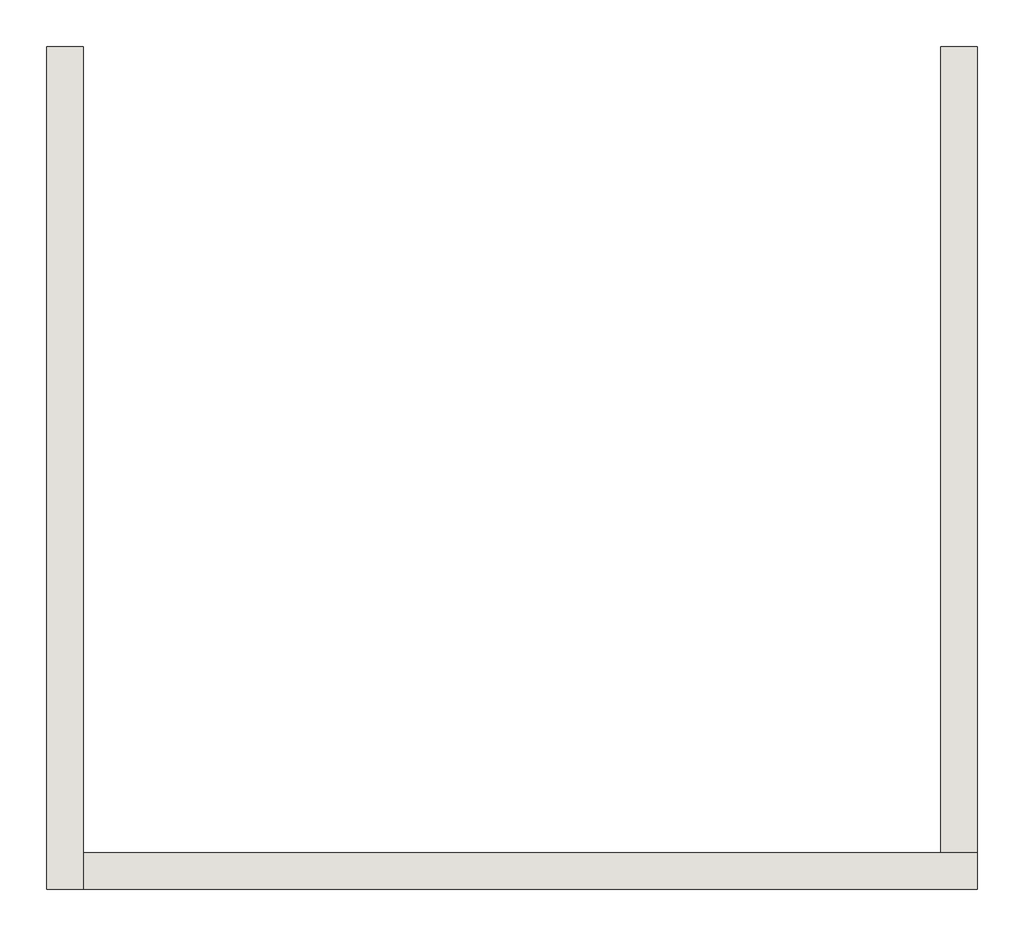
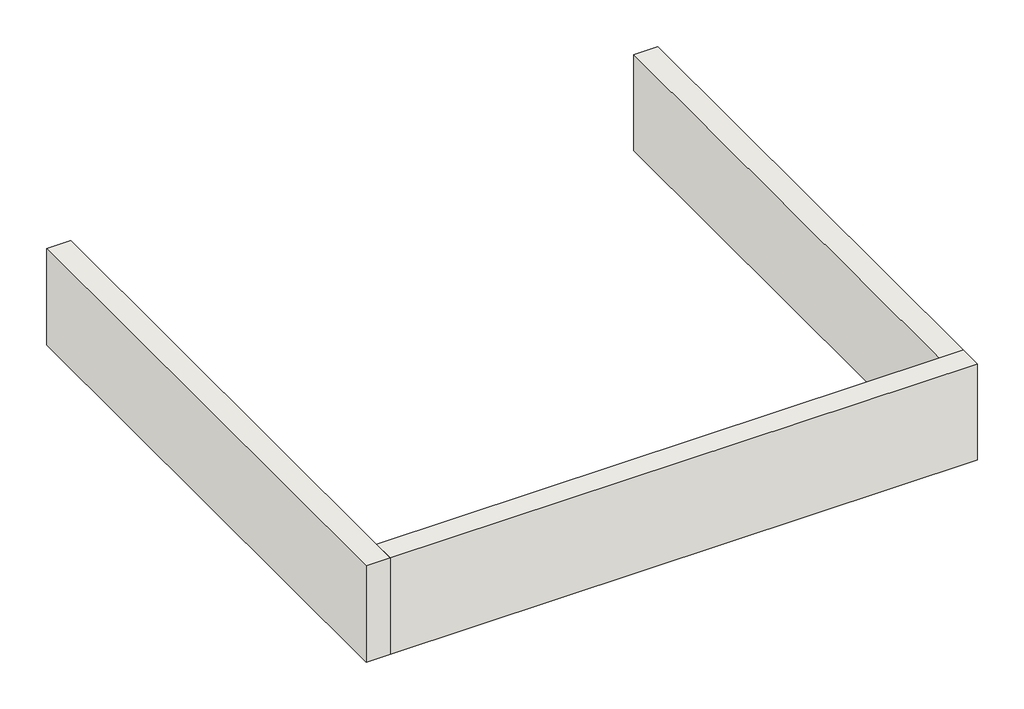
# One storey: 3 walls.
"""IFC4 building model written with IfcOpenShell, lengths in millimetres."""

from ifc_helpers import new_model, si_unit, frame, origin, place, context, project, spatial, polyline, outline, extrude, faceted_brep, element, save

model = new_model("IFC4")

# Units and contexts
model_context = context("Model", 3, world=origin())
ifc_project = project(units=[si_unit("LENGTHUNIT", "METRE", prefix="MILLI")], contexts=[model_context])

# Site, building, storey
site = spatial("IfcSite", under=ifc_project)
building = spatial("IfcBuilding", under=site)
storey = spatial("IfcBuildingStorey", under=building, Elevation=16002.0)

# Walls
placement = place(None, origin())
element("IfcWall", 1, ObjectType="5\"", at=placement, inside=storey, context=model_context, shape_type="Brep", body=[
    faceted_brep([(907.1132171, -5589.2354899, 15468.6), (907.1132171, -5462.2354899, 15468.6), (907.1132171, -2688.7252054, 15468.6), (907.1132171, -2688.7252054, 16002.0), (907.1132171, -5462.2354899, 16002.0), (907.1132171, -5589.2354899, 16002.0), (780.1132171, -5589.2354899, 15468.6), (780.1132171, -5589.2354899, 16002.0), (780.1132171, -2688.7252054, 16002.0), (780.1132171, -2688.7252054, 15468.6)], [[[0, 1, 2, 3, 4, 5]], [[6, 7, 8, 9]], [[2, 1, 0, 6, 9]], [[3, 2, 9, 8]], [[5, 4, 3, 8, 7]], [[0, 5, 7, 6]]]),
])
element("IfcWall", 2, ObjectType="5\"", at=placement, inside=storey, context=model_context, shape_type="SweptSolid", body=[
    extrude(outline(polyline([(3983.5941077, -2688.7252054), (3983.5941077, -5462.2354899), (3856.5941077, -5462.2354899), (3856.5941077, -2688.7252054), (3983.5941077, -2688.7252054)])), frame((0.0, 0.0, 15468.6), z_axis=(0.0, 0.0, 1.0), x_axis=(1.0, 0.0, 0.0)), (0.0, 0.0, 1.0), 533.4),
])
element("IfcWall", 3, ObjectType="5\"", at=placement, inside=storey, context=model_context, shape_type="Brep", body=[
    faceted_brep([(3983.5941077, -5462.2354899, 15468.6), (3856.5941077, -5462.2354899, 15468.6), (907.1132171, -5462.2354899, 15468.6), (907.1132171, -5462.2354899, 16002.0), (3856.5941077, -5462.2354899, 16002.0), (3983.5941077, -5462.2354899, 16002.0), (3983.5941077, -5589.2354899, 15468.6), (3983.5941077, -5589.2354899, 16002.0), (907.1132171, -5589.2354899, 16002.0), (907.1132171, -5589.2354899, 15468.6)], [[[0, 1, 2, 3, 4, 5]], [[6, 7, 8, 9]], [[2, 1, 0, 6, 9]], [[5, 4, 3, 8, 7]], [[3, 2, 9, 8]], [[0, 5, 7, 6]]]),
])

save(model, "model.ifc")

# Revit data of these elements
# Type "5\""
#   Keynote = "F10"
#   Layers, outside or top first: 0' - 5" "Concrete" (function 1)
# Element 1 (IfcWall, "5\"")
#   built-in parameter 1001111 = -1' - 9"
#   Top Offset = 0' - 0"
#   Base Offset = -1' - 9"
#   Unconnected Height = 1' - 9"
#   wall height = 1' - 9"
#   Phase Created = New Construction
#   Base Constraint = TOP LEV.
#   Materials on its faces: "Concrete", "Blue"
# Element 2 (IfcWall, "5\"")
#   built-in parameter 1001111 = -1' - 9"
#   Top Offset = 0' - 0"
#   Base Offset = -1' - 9"
#   Unconnected Height = 1' - 9"
#   wall height = 1' - 9"
#   Phase Created = New Construction
#   Base Constraint = TOP LEV.
#   Materials on its faces: "Concrete", "Clad - White"
# Element 3 (IfcWall, "5\"")
#   built-in parameter 1001111 = -1' - 9"
#   Top Offset = 0' - 0"
#   Base Offset = -1' - 9"
#   Unconnected Height = 1' - 9"
#   wall height = 1' - 9"
#   Phase Created = New Construction
#   Base Constraint = TOP LEV.
#   Materials on its faces: "Concrete", "Blue", "Clad - White"
# Materials
#   "Concrete": class "Concrete", colour RGB 120 120 120, transparency 0, Description = "Portland Cement Concrete", Cost = 0
#   "Blue": class "Generic", colour RGB 0 43 85, transparency 0, Cost = 0
#   "Clad - White": class "Wood", colour RGB 242 242 238, transparency 0, Cost = 0
